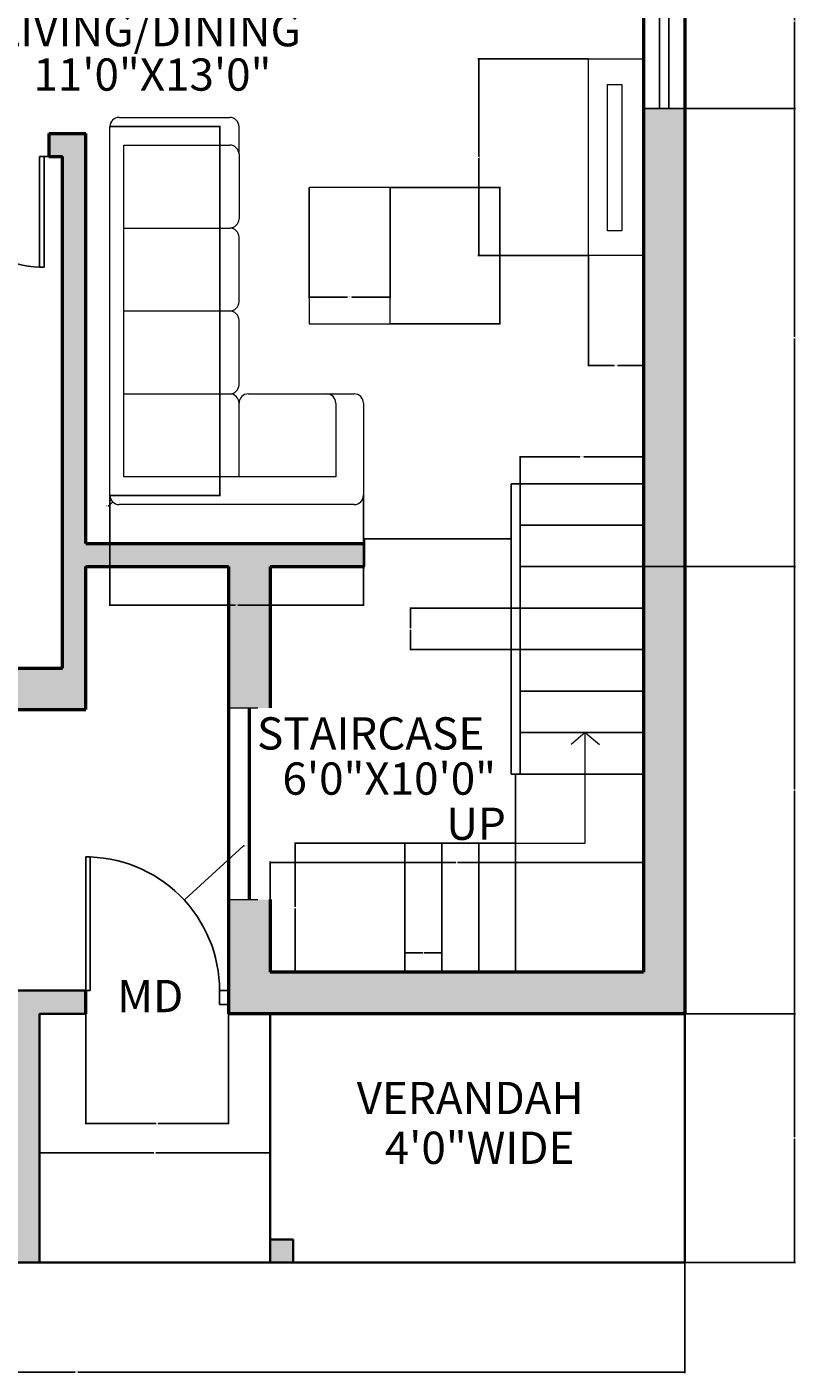
# Model space of a CAD drawing. Units: inches. Extents: x 2715 to 3027, y 1777 to 2287.
# Tile 2 of 4: x 2860 to 3027, y 1777 to 2069. Entities that reach past the tile are written whole.
import ezdxf

# ---------------------------------------------------------------- set-up
doc = ezdxf.new("R2010")
doc.units = ezdxf.units.IN
doc.linetypes.add('DASHED2', pattern=[9.525, 6.35, -3.175])
for name, color, linetype, lineweight in [('A-ANNO-DIMS', 2, 'Continuous', 18), ('A-ANNO-SYMB', 7, 'Continuous', 18), ('A-ANNO-TEXT', 2, 'Continuous', 18), ('A-AREA-IDEN', 2, 'Continuous', 18), ('A-DOOR', 111, 'Continuous', 25), ('A-EQPM', 57, 'Continuous', 18), ('A-FLOR-STRS', 7, 'Continuous', 25), ('A-FURN', 201, 'Continuous', 18), ('A-GLAZ', 40, 'Continuous', 25), ('A-WALL', 7, 'Continuous', 50), ('A-WALL-HIDN', 255, 'DASHED2', 18), ('A-WALL-PATT', 252, 'Continuous', 13), ('C-SITE', 7, 'Continuous', 35)]:
    doc.layers.add(name, color=color, linetype=linetype, lineweight=lineweight)
doc.styles.get("Standard").update_dxf_attribs({"font": 'arial.ttf'})
doc.dimstyles.get("Standard").update_dxf_attribs({"dimtxt": 0.18, "dimasz": 0.18, "dimexe": 0.18, "dimexo": 0.0625, "dimgap": 0.09, "dimtad": 0, "dimtih": 1, "dimtoh": 1, "dimdec": 4, "dimzin": 0, "dimdsep": 46, "dimtxsty": 'Standard', "dimcen": 0.09, "dimadec": 0, "dimazin": 0, "dimtfac": 1, "dimtdec": 4, "dimtofl": 0, "dimtmove": 0, "dimatfit": 3, "dimfxl": 1, "dimtolj": 1, "dimtzin": 0, "dimarcsym": 0})

# ---------------------------------------------------------------- blocks, each defined once
blk = doc.blocks.new('*D25')
at = {"layer": 'A-ANNO-DIMS', "color": 0, "lineweight": -2, "transparency": 16777216}
for p, q in [((2738.92, 1801.28), (2738.92, 1777.36)), ((3002.92, 1801.28), (3002.92, 1777.36)), ((2739.1, 1777.54), (2870.63, 1777.54)), ((3002.74, 1777.54), (2871.21, 1777.54))]:
    blk.add_line(p, q, dxfattribs=at)
at = {"layer": 'A-ANNO-DIMS', "color": 0, "transparency": 16777216}
for points in [[(2739.1, 1777.57), (2739.1, 1777.51), (2738.92, 1777.54)], [(3002.74, 1777.57), (3002.74, 1777.51), (3002.92, 1777.54)]]:
    blk.add_solid(points, dxfattribs=at)
at = {"layer": 'Defpoints', "color": 0, "transparency": 16777216}
for p in [(2738.92, 1801.34), (3002.92, 1801.34), (3002.92, 1777.54)]:
    blk.add_point(p, dxfattribs=at)
at = {"layer": 'A-ANNO-DIMS', "color": 0, "transparency": 16777216, "insert": (2870.92, 1777.54), "char_height": 0.18, "attachment_point": 5}
blk.add_mtext('\\A1;264', dxfattribs=at)
blk = doc.blocks.new('*D27')
at = {"layer": 'A-ANNO-DIMS', "color": 0, "lineweight": -2, "transparency": 16777216}
for p, q in [((3002.98, 1855.34), (3026.9, 1855.34)), ((3026.72, 1855.16), (3026.72, 1828.52)), ((3026.72, 1801.52), (3026.72, 1828.16)), ((3002.98, 1801.34), (3026.9, 1801.34))]:
    blk.add_line(p, q, dxfattribs=at)
at = {"layer": 'A-ANNO-DIMS', "color": 0, "transparency": 16777216}
for points in [[(3026.69, 1855.16), (3026.75, 1855.16), (3026.72, 1855.34)], [(3026.69, 1801.52), (3026.75, 1801.52), (3026.72, 1801.34)]]:
    blk.add_solid(points, dxfattribs=at)
at = {"layer": 'Defpoints', "color": 0, "transparency": 16777216}
for p in [(3002.92, 1855.34), (3026.72, 1855.34), (3002.92, 1801.34)]:
    blk.add_point(p, dxfattribs=at)
at = {"layer": 'A-ANNO-DIMS', "color": 0, "transparency": 16777216, "insert": (3026.72, 1828.34), "char_height": 0.18, "attachment_point": 5}
blk.add_mtext('\\A1;54', dxfattribs=at)
blk = doc.blocks.new('*D28')
at = {"layer": 'A-ANNO-DIMS', "color": 0, "lineweight": -2, "transparency": 16777216}
for p, q in [((2993.98, 1952.34), (3026.9, 1952.34)), ((3026.72, 1952.16), (3026.72, 1904.02)), ((3026.72, 1855.52), (3026.72, 1903.66)), ((3002.98, 1855.34), (3026.9, 1855.34))]:
    blk.add_line(p, q, dxfattribs=at)
at = {"layer": 'A-ANNO-DIMS', "color": 0, "transparency": 16777216}
for points in [[(3026.69, 1952.16), (3026.75, 1952.16), (3026.72, 1952.34)], [(3026.69, 1855.52), (3026.75, 1855.52), (3026.72, 1855.34)]]:
    blk.add_solid(points, dxfattribs=at)
at = {"layer": 'Defpoints', "color": 0, "transparency": 16777216}
for p in [(2993.92, 1952.34), (3026.72, 1952.34), (3002.92, 1855.34)]:
    blk.add_point(p, dxfattribs=at)
at = {"layer": 'A-ANNO-DIMS', "color": 0, "transparency": 16777216, "insert": (3026.72, 1903.84), "char_height": 0.18, "attachment_point": 5}
blk.add_mtext('\\A1;97', dxfattribs=at)
blk = doc.blocks.new('*D29')
at = {"layer": 'A-ANNO-DIMS', "color": 0, "lineweight": -2, "transparency": 16777216}
for p, q in [((3002.98, 2051.72), (3026.9, 2051.72)), ((3026.72, 2051.54), (3026.72, 2002.21)), ((3026.72, 1952.52), (3026.72, 2001.85)), ((2993.98, 1952.34), (3026.9, 1952.34))]:
    blk.add_line(p, q, dxfattribs=at)
at = {"layer": 'A-ANNO-DIMS', "color": 0, "transparency": 16777216}
for points in [[(3026.69, 2051.54), (3026.75, 2051.54), (3026.72, 2051.72)], [(3026.69, 1952.52), (3026.75, 1952.52), (3026.72, 1952.34)]]:
    blk.add_solid(points, dxfattribs=at)
at = {"layer": 'Defpoints', "color": 0, "transparency": 16777216}
for p in [(3002.92, 2051.72), (3026.72, 2051.72), (2993.92, 1952.34)]:
    blk.add_point(p, dxfattribs=at)
at = {"layer": 'A-ANNO-DIMS', "color": 0, "transparency": 16777216, "insert": (3026.72, 2002.03), "char_height": 0.18, "attachment_point": 5}
blk.add_mtext('\\A1;99.38', dxfattribs=at)
blk = doc.blocks.new('*D30')
at = {"layer": 'A-ANNO-DIMS', "color": 0, "lineweight": -2, "transparency": 16777216}
for p, q in [((3002.98, 2089.72), (3026.9, 2089.72)), ((3026.72, 2089.54), (3026.72, 2070.9)), ((3026.72, 2051.9), (3026.72, 2070.54)), ((3002.98, 2051.72), (3026.9, 2051.72))]:
    blk.add_line(p, q, dxfattribs=at)
at = {"layer": 'A-ANNO-DIMS', "color": 0, "transparency": 16777216}
for points in [[(3026.69, 2089.54), (3026.75, 2089.54), (3026.72, 2089.72)], [(3026.69, 2051.9), (3026.75, 2051.9), (3026.72, 2051.72)]]:
    blk.add_solid(points, dxfattribs=at)
at = {"layer": 'Defpoints', "color": 0, "transparency": 16777216}
for p in [(3002.92, 2089.72), (3026.72, 2089.72), (3002.92, 2051.72)]:
    blk.add_point(p, dxfattribs=at)
at = {"layer": 'A-ANNO-DIMS', "color": 0, "transparency": 16777216, "insert": (3026.72, 2070.72), "char_height": 0.18, "attachment_point": 5}
blk.add_mtext('\\A1;38', dxfattribs=at)
blk = doc.blocks.new('*D45')
at = {"layer": 'A-ANNO-DIMS', "color": 0, "lineweight": -2, "transparency": 16777216}
for p, q in [((2862.92, 1801.4), (2862.92, 1825.33)), ((2863.1, 1825.15), (2887.7, 1825.15)), ((2912.74, 1825.15), (2888.13, 1825.15)), ((2912.92, 1801.4), (2912.92, 1825.33))]:
    blk.add_line(p, q, dxfattribs=at)
at = {"layer": 'A-ANNO-DIMS', "color": 0, "transparency": 16777216}
for points in [[(2863.1, 1825.18), (2863.1, 1825.12), (2862.92, 1825.15)], [(2912.74, 1825.18), (2912.74, 1825.12), (2912.92, 1825.15)]]:
    blk.add_solid(points, dxfattribs=at)
at = {"layer": 'Defpoints', "color": 0, "transparency": 16777216}
for p in [(2912.92, 1825.15), (2862.92, 1801.34), (2912.92, 1801.34)]:
    blk.add_point(p, dxfattribs=at)
at = {"layer": 'A-ANNO-DIMS', "color": 0, "transparency": 16777216, "insert": (2887.92, 1825.15), "char_height": 0.18, "attachment_point": 5}
blk.add_mtext('\\A1;50', dxfattribs=at)
blk = doc.blocks.new('*D46')
at = {"layer": 'A-ANNO-DIMS', "color": 0, "lineweight": -2, "transparency": 16777216}
for p, q in [((2912.92, 1864.4), (2912.92, 1888.33)), ((2913.1, 1888.15), (2953.21, 1888.15)), ((2993.74, 1888.15), (2953.62, 1888.15)), ((2993.92, 1864.4), (2993.92, 1888.33))]:
    blk.add_line(p, q, dxfattribs=at)
at = {"layer": 'A-ANNO-DIMS', "color": 0, "transparency": 16777216}
for points in [[(2913.1, 1888.18), (2913.1, 1888.12), (2912.92, 1888.15)], [(2993.74, 1888.18), (2993.74, 1888.12), (2993.92, 1888.15)]]:
    blk.add_solid(points, dxfattribs=at)
at = {"layer": 'Defpoints', "color": 0, "transparency": 16777216}
for p in [(2993.92, 1888.15), (2912.92, 1864.34), (2993.92, 1864.34)]:
    blk.add_point(p, dxfattribs=at)
at = {"layer": 'A-ANNO-DIMS', "color": 0, "transparency": 16777216, "insert": (2953.42, 1888.15), "char_height": 0.18, "attachment_point": 5}
blk.add_mtext('\\A1;81', dxfattribs=at)
blk = doc.blocks.new('*D50')
at = {"layer": 'A-ANNO-DIMS', "color": 0, "lineweight": -2, "transparency": 16777216}
for p, q in [((2872.92, 1855.28), (2872.92, 1831.36)), ((2903.92, 1855.28), (2903.92, 1831.36)), ((2873.1, 1831.54), (2888.21, 1831.54)), ((2903.74, 1831.54), (2888.62, 1831.54))]:
    blk.add_line(p, q, dxfattribs=at)
at = {"layer": 'A-ANNO-DIMS', "color": 0, "transparency": 16777216}
for points in [[(2873.1, 1831.57), (2873.1, 1831.51), (2872.92, 1831.54)], [(2903.74, 1831.57), (2903.74, 1831.51), (2903.92, 1831.54)]]:
    blk.add_solid(points, dxfattribs=at)
at = {"layer": 'Defpoints', "color": 0, "transparency": 16777216}
for p in [(2872.92, 1855.34), (2903.92, 1855.34), (2872.92, 1831.54)]:
    blk.add_point(p, dxfattribs=at)
at = {"layer": 'A-ANNO-DIMS', "color": 0, "transparency": 16777216, "insert": (2888.42, 1831.54), "char_height": 0.18, "attachment_point": 5}
blk.add_mtext('\\A1;31', dxfattribs=at)
blk = doc.blocks.new('*D62')
at = {"layer": 'A-ANNO-DIMS', "color": 0, "lineweight": -2, "transparency": 16777216}
for p, q in [((2878.17, 1967.75), (2878.17, 1943.83)), ((2933.17, 1967.75), (2933.17, 1943.83)), ((2878.35, 1944.01), (2905.45, 1944.01)), ((2932.99, 1944.01), (2905.89, 1944.01))]:
    blk.add_line(p, q, dxfattribs=at)
at = {"layer": 'A-ANNO-DIMS', "color": 0, "transparency": 16777216}
for points in [[(2878.35, 1944.04), (2878.35, 1943.98), (2878.17, 1944.01)], [(2932.99, 1944.04), (2932.99, 1943.98), (2933.17, 1944.01)]]:
    blk.add_solid(points, dxfattribs=at)
at = {"layer": 'Defpoints', "color": 0, "transparency": 16777216}
for p in [(2878.17, 1967.81), (2933.17, 1967.81), (2878.17, 1944.01)]:
    blk.add_point(p, dxfattribs=at)
at = {"layer": 'A-ANNO-DIMS', "color": 0, "transparency": 16777216, "insert": (2905.67, 1944.01), "char_height": 0.18, "attachment_point": 5}
blk.add_mtext('\\A1;55', dxfattribs=at)
blk = doc.blocks.new('*D63')
at = {"layer": 'A-ANNO-DIMS', "color": 0, "lineweight": -2, "transparency": 16777216}
for p, q in [((2878.24, 2047.81), (2902.16, 2047.81)), ((2901.98, 2047.63), (2901.98, 2008)), ((2901.98, 1967.99), (2901.98, 2007.63)), ((2878.24, 1967.81), (2902.16, 1967.81))]:
    blk.add_line(p, q, dxfattribs=at)
at = {"layer": 'A-ANNO-DIMS', "color": 0, "transparency": 16777216}
for points in [[(2901.95, 2047.63), (2902.01, 2047.63), (2901.98, 2047.81)], [(2901.95, 1967.99), (2902.01, 1967.99), (2901.98, 1967.81)]]:
    blk.add_solid(points, dxfattribs=at)
at = {"layer": 'Defpoints', "color": 0, "transparency": 16777216}
for p in [(2878.17, 2047.81), (2878.17, 1967.81), (2901.98, 1967.81)]:
    blk.add_point(p, dxfattribs=at)
at = {"layer": 'A-ANNO-DIMS', "color": 0, "transparency": 16777216, "insert": (2901.98, 2007.81), "char_height": 0.18, "attachment_point": 5}
blk.add_mtext('\\A1;80', dxfattribs=at)
blk = doc.blocks.new('*D67')
at = {"layer": 'A-ANNO-DIMS', "color": 0, "lineweight": -2, "transparency": 16777216}
for p, q in [((2939.02, 2034.61), (2962.94, 2034.61)), ((2962.76, 2034.43), (2962.76, 2020.01)), ((2962.76, 2005.23), (2962.76, 2019.65)), ((2939.02, 2005.05), (2962.94, 2005.05))]:
    blk.add_line(p, q, dxfattribs=at)
at = {"layer": 'A-ANNO-DIMS', "color": 0, "transparency": 16777216}
for points in [[(2962.73, 2034.43), (2962.79, 2034.43), (2962.76, 2034.61)], [(2962.73, 2005.23), (2962.79, 2005.23), (2962.76, 2005.05)]]:
    blk.add_solid(points, dxfattribs=at)
at = {"layer": 'Defpoints', "color": 0, "transparency": 16777216}
for p in [(2938.95, 2034.61), (2938.95, 2005.05), (2962.76, 2005.05)]:
    blk.add_point(p, dxfattribs=at)
at = {"layer": 'A-ANNO-DIMS', "color": 0, "transparency": 16777216, "insert": (2962.76, 2019.83), "char_height": 0.18, "attachment_point": 5}
blk.add_mtext('\\A1;29.57', dxfattribs=at)
blk = doc.blocks.new('*D68')
at = {"layer": 'A-ANNO-DIMS', "color": 0, "lineweight": -2, "transparency": 16777216}
for p, q in [((2921.42, 2034.55), (2921.42, 2010.63)), ((2938.95, 2034.55), (2938.95, 2010.63)), ((2921.6, 2010.81), (2929.73, 2010.81)), ((2938.77, 2010.81), (2930.64, 2010.81))]:
    blk.add_line(p, q, dxfattribs=at)
at = {"layer": 'A-ANNO-DIMS', "color": 0, "transparency": 16777216}
for points in [[(2921.6, 2010.84), (2921.6, 2010.78), (2921.42, 2010.81)], [(2938.77, 2010.84), (2938.77, 2010.78), (2938.95, 2010.81)]]:
    blk.add_solid(points, dxfattribs=at)
at = {"layer": 'Defpoints', "color": 0, "transparency": 16777216}
for p in [(2921.42, 2034.61), (2938.95, 2034.61), (2921.42, 2010.81)]:
    blk.add_point(p, dxfattribs=at)
at = {"layer": 'A-ANNO-DIMS', "color": 0, "transparency": 16777216, "insert": (2930.19, 2010.81), "char_height": 0.18, "attachment_point": 5}
blk.add_mtext('\\A1;17.537', dxfattribs=at)
blk = doc.blocks.new('*D69')
at = {"layer": 'A-ANNO-DIMS', "color": 0, "lineweight": -2, "transparency": 16777216}
for p, q in [((2981.91, 2062.54), (2957.99, 2062.54)), ((2958.17, 2062.36), (2958.17, 2041.36)), ((2958.17, 2020.01), (2958.17, 2041)), ((2981.91, 2019.83), (2957.99, 2019.83))]:
    blk.add_line(p, q, dxfattribs=at)
at = {"layer": 'A-ANNO-DIMS', "color": 0, "transparency": 16777216}
for points in [[(2958.14, 2062.36), (2958.2, 2062.36), (2958.17, 2062.54)], [(2958.14, 2020.01), (2958.2, 2020.01), (2958.17, 2019.83)]]:
    blk.add_solid(points, dxfattribs=at)
at = {"layer": 'Defpoints', "color": 0, "transparency": 16777216}
for p in [(2958.17, 2062.54), (2981.97, 2062.54), (2981.97, 2019.83)]:
    blk.add_point(p, dxfattribs=at)
at = {"layer": 'A-ANNO-DIMS', "color": 0, "transparency": 16777216, "insert": (2958.17, 2041.18), "char_height": 0.18, "attachment_point": 5}
blk.add_mtext('\\A1;42.71', dxfattribs=at)
blk = doc.blocks.new('*D70')
at = {"layer": 'A-ANNO-DIMS', "color": 0, "lineweight": -2, "transparency": 16777216}
for p, q in [((2981.97, 2019.77), (2981.97, 1995.84)), ((2993.92, 2019.77), (2993.92, 1995.84)), ((2982.15, 1996.02), (2987.56, 1996.02)), ((2993.74, 1996.02), (2988.33, 1996.02))]:
    blk.add_line(p, q, dxfattribs=at)
at = {"layer": 'A-ANNO-DIMS', "color": 0, "transparency": 16777216}
for points in [[(2982.15, 1996.05), (2982.15, 1995.99), (2981.97, 1996.02)], [(2993.74, 1996.05), (2993.74, 1995.99), (2993.92, 1996.02)]]:
    blk.add_solid(points, dxfattribs=at)
at = {"layer": 'Defpoints', "color": 0, "transparency": 16777216}
for p in [(2981.97, 2019.83), (2993.92, 2019.83), (2981.97, 1996.02)]:
    blk.add_point(p, dxfattribs=at)
at = {"layer": 'A-ANNO-DIMS', "color": 0, "transparency": 16777216, "insert": (2987.95, 1996.02), "char_height": 0.18, "attachment_point": 5}
blk.add_mtext('\\A1;11.94', dxfattribs=at)
blk = doc.blocks.new('*D71')
at = {"layer": 'A-ANNO-DIMS', "color": 0, "lineweight": -2, "transparency": 16777216}
for p, q in [((2967.18, 1952.4), (2967.18, 1976.33)), ((2967.36, 1976.15), (2980.08, 1976.15)), ((2993.74, 1976.15), (2981.01, 1976.15)), ((2993.92, 1952.4), (2993.92, 1976.33))]:
    blk.add_line(p, q, dxfattribs=at)
at = {"layer": 'A-ANNO-DIMS', "color": 0, "transparency": 16777216}
for points in [[(2967.36, 1976.18), (2967.36, 1976.12), (2967.18, 1976.15)], [(2993.74, 1976.18), (2993.74, 1976.12), (2993.92, 1976.15)]]:
    blk.add_solid(points, dxfattribs=at)
at = {"layer": 'Defpoints', "color": 0, "transparency": 16777216}
for p in [(2993.92, 1976.15), (2967.18, 1952.34), (2993.92, 1952.34)]:
    blk.add_point(p, dxfattribs=at)
at = {"layer": 'A-ANNO-DIMS', "color": 0, "transparency": 16777216, "insert": (2980.55, 1976.15), "char_height": 0.18, "attachment_point": 5}
blk.add_mtext('\\A1;26.733', dxfattribs=at)
blk = doc.blocks.new('*D72')
at = {"layer": 'A-ANNO-DIMS', "color": 0, "lineweight": -2, "transparency": 16777216}
for p, q in [((2967.12, 1943.34), (2943.2, 1943.34)), ((2943.38, 1943.16), (2943.38, 1939.02)), ((2943.38, 1934.52), (2943.38, 1938.66)), ((2967.12, 1934.34), (2943.2, 1934.34))]:
    blk.add_line(p, q, dxfattribs=at)
at = {"layer": 'A-ANNO-DIMS', "color": 0, "transparency": 16777216}
for points in [[(2943.35, 1943.16), (2943.41, 1943.16), (2943.38, 1943.34)], [(2943.35, 1934.52), (2943.41, 1934.52), (2943.38, 1934.34)]]:
    blk.add_solid(points, dxfattribs=at)
at = {"layer": 'Defpoints', "color": 0, "transparency": 16777216}
for p in [(2943.38, 1943.34), (2967.18, 1943.34), (2967.18, 1934.34)]:
    blk.add_point(p, dxfattribs=at)
at = {"layer": 'A-ANNO-DIMS', "color": 0, "transparency": 16777216, "insert": (2943.38, 1938.84), "char_height": 0.18, "attachment_point": 5}
blk.add_mtext('\\A1;9', dxfattribs=at)
blk = doc.blocks.new('*D73')
at = {"layer": 'A-ANNO-DIMS', "color": 0, "lineweight": -2, "transparency": 16777216}
for p, q in [((2942.18, 1892.28), (2942.18, 1868.36)), ((2950.18, 1892.28), (2950.18, 1868.36)), ((2942.36, 1868.54), (2946.03, 1868.54)), ((2950, 1868.54), (2946.33, 1868.54))]:
    blk.add_line(p, q, dxfattribs=at)
at = {"layer": 'A-ANNO-DIMS', "color": 0, "transparency": 16777216}
for points in [[(2942.36, 1868.57), (2942.36, 1868.51), (2942.18, 1868.54)], [(2950, 1868.57), (2950, 1868.51), (2950.18, 1868.54)]]:
    blk.add_solid(points, dxfattribs=at)
at = {"layer": 'Defpoints', "color": 0, "transparency": 16777216}
for p in [(2942.18, 1892.34), (2950.18, 1892.34), (2942.18, 1868.54)]:
    blk.add_point(p, dxfattribs=at)
at = {"layer": 'A-ANNO-DIMS', "color": 0, "transparency": 16777216, "insert": (2946.18, 1868.54), "char_height": 0.18, "attachment_point": 5}
blk.add_mtext('\\A1;8', dxfattribs=at)
blk = doc.blocks.new('*D74')
at = {"layer": 'A-ANNO-DIMS', "color": 0, "lineweight": -2, "transparency": 16777216}
for p, q in [((2942.12, 1892.34), (2918.2, 1892.34)), ((2918.38, 1892.16), (2918.38, 1878.52)), ((2918.38, 1864.52), (2918.38, 1878.16)), ((2942.12, 1864.34), (2918.2, 1864.34))]:
    blk.add_line(p, q, dxfattribs=at)
at = {"layer": 'A-ANNO-DIMS', "color": 0, "transparency": 16777216}
for points in [[(2918.35, 1892.16), (2918.41, 1892.16), (2918.38, 1892.34)], [(2918.35, 1864.52), (2918.41, 1864.52), (2918.38, 1864.34)]]:
    blk.add_solid(points, dxfattribs=at)
at = {"layer": 'Defpoints', "color": 0, "transparency": 16777216}
for p in [(2918.38, 1892.34), (2942.18, 1892.34), (2942.18, 1864.34)]:
    blk.add_point(p, dxfattribs=at)
at = {"layer": 'A-ANNO-DIMS', "color": 0, "transparency": 16777216, "insert": (2918.38, 1878.34), "char_height": 0.18, "attachment_point": 5}
blk.add_mtext('\\A1;28', dxfattribs=at)
blk = doc.blocks.new('*D75')
at = {"layer": 'A-ANNO-DIMS', "color": 0, "lineweight": -2, "transparency": 16777216}
for p, q in [((2907.14, 1891.73), (2894.45, 1880.09)), ((2907.32, 1891.73), (2907.14, 1891.73)), ((2872.87, 1860.36), (2873.05, 1860.36)), ((2872.96, 1860.27), (2872.96, 1860.45))]:
    blk.add_line(p, q, dxfattribs=at)
at = {"layer": 'A-ANNO-DIMS', "color": 0, "transparency": 16777216}
blk.add_solid([(2894.43, 1880.11), (2894.47, 1880.07), (2894.32, 1879.97)], dxfattribs=at)
at = {"layer": 'Defpoints', "color": 0, "transparency": 16777216}
for p in [(2894.32, 1879.97), (2872.96, 1860.36)]:
    blk.add_point(p, dxfattribs=at)
at = {"layer": 'A-ANNO-DIMS', "color": 0, "transparency": 16777216, "insert": (2907.62, 1891.73), "char_height": 0.18, "attachment_point": 5}
blk.add_mtext('\\A1;R29', dxfattribs=at)
blk = doc.blocks.new('*D77')
at = {"layer": 'A-ANNO-DIMS', "color": 0, "lineweight": -2, "transparency": 16777216}
for p, q in [((2863.69, 2041.32), (2863.87, 2041.32)), ((2863.78, 2041.23), (2863.78, 2041.41)), ((2834.78, 2016.15), (2845.52, 2025.48)), ((2834.6, 2016.15), (2834.78, 2016.15))]:
    blk.add_line(p, q, dxfattribs=at)
at = {"layer": 'A-ANNO-DIMS', "color": 0, "transparency": 16777216}
blk.add_solid([(2845.5, 2025.5), (2845.54, 2025.45), (2845.66, 2025.59)], dxfattribs=at)
at = {"layer": 'Defpoints', "color": 0, "transparency": 16777216}
for p in [(2863.78, 2041.32), (2845.66, 2025.59)]:
    blk.add_point(p, dxfattribs=at)
at = {"layer": 'A-ANNO-DIMS', "color": 0, "transparency": 16777216, "insert": (2834.11, 2016.15), "char_height": 0.18, "attachment_point": 5}
blk.add_mtext('\\A1;3X R24', dxfattribs=at)
blk = doc.blocks.new('*D79')
at = {"layer": 'A-ANNO-DIMS', "color": 0, "lineweight": -2, "transparency": 16777216}
for p, q in [((2877.94, 1965.52), (2878.65, 1966.25)), ((2880.08, 1967.81), (2880.26, 1967.81)), ((2880.17, 1967.72), (2880.17, 1967.9)), ((2877.76, 1965.52), (2877.94, 1965.52))]:
    blk.add_line(p, q, dxfattribs=at)
at = {"layer": 'A-ANNO-DIMS', "color": 0, "transparency": 16777216}
blk.add_solid([(2878.63, 1966.27), (2878.68, 1966.23), (2878.78, 1966.38)], dxfattribs=at)
at = {"layer": 'Defpoints', "color": 0, "transparency": 16777216}
for p in [(2878.78, 1966.38), (2880.17, 1967.81)]:
    blk.add_point(p, dxfattribs=at)
at = {"layer": 'A-ANNO-DIMS', "color": 0, "transparency": 16777216, "insert": (2877.53, 1965.52), "char_height": 0.18, "attachment_point": 5}
blk.add_mtext('\\A1;R2', dxfattribs=at)

msp = doc.modelspace()

# ---------------------------------------------------------------- hatches: boundary and pattern name
at = {"layer": 'A-WALL-PATT'}
h = msp.add_hatch(color=256, dxfattribs=at)
h.dxf.hatch_style = 1
h.paths.add_polyline_path([(3002.9159, 2051.722), (2993.9159, 2051.722), (2993.9159, 2019.8298), (2993.9159, 1864.3404), (2912.9159, 1864.3404), (2912.9159, 1880.0932), (2903.9159, 1880.0932), (2903.9159, 1864.3404), (2903.9159, 1855.3404), (3002.9159, 1855.3404)])
h = msp.add_hatch(color=256, dxfattribs=at)
h.dxf.hatch_style = 1
h.paths.add_polyline_path([(2872.9159, 2046.3404), (2864.9159, 2046.3404), (2864.9159, 2041.3404), (2867.9159, 2041.3404), (2867.9159, 1930.3404), (2829.9565, 1930.3404), (2829.9565, 1921.3404), (2872.9159, 1921.3404), (2872.9159, 1952.3404), (2903.9159, 1952.3404), (2903.9159, 1921.6914), (2912.9159, 1921.6914), (2912.9159, 1952.3404), (2933.4159, 1952.3404), (2933.4159, 1957.3404), (2872.9159, 1957.3404)])
h = msp.add_hatch(color=256, dxfattribs=at)
h.dxf.hatch_style = 1
h.paths.add_polyline_path([(2862.9159, 1855.3404), (2872.9159, 1855.3404), (2872.9159, 1860.3404), (2857.9159, 1860.3404), (2857.9159, 1806.3404), (2852.094, 1806.3404), (2852.094, 1801.3404), (2857.9159, 1801.3404), (2862.9159, 1801.3404)])
h = msp.add_hatch(color=256, dxfattribs=at)
h.dxf.hatch_style = 1
h.paths.add_polyline_path([(2917.9159, 1806.3404), (2912.9159, 1806.3404), (2912.9159, 1801.3404), (2917.9159, 1801.3404)])

# ---------------------------------------------------------------- linework, layer by layer
at = {"layer": 'A-ANNO-SYMB'}
for p, q in [((2981.2868, 1916.3404), (2978.2226, 1913.7692)), ((2981.2868, 1892.3404), (2981.2868, 1916.3404)), ((2981.2868, 1916.3404), (2984.3509, 1913.7692)), ((2966.1833, 1892.3404), (2981.2868, 1892.3404))]:
    msp.add_line(p, q, dxfattribs=at)
at = {"layer": 'A-DOOR'}
for p, q in [((2862.9159, 2017.3404), (2862.9159, 2041.3404)), ((2862.9159, 2041.3404), (2863.9159, 2041.3404)), ((2864.9159, 2041.3404), (2863.9159, 2041.3404)), ((2863.9159, 2041.3404), (2863.9159, 2017.3404)), ((2863.9159, 2017.3404), (2862.9159, 2017.3404)), ((2872.9159, 1860.3404), (2872.9159, 1889.3404)), ((2872.9159, 1889.3404), (2873.9159, 1889.3404)), ((2873.9159, 1889.3404), (2873.9159, 1860.3404)), ((2873.9159, 1860.3404), (2872.9159, 1860.3404)), ((2901.9159, 1860.3404), (2903.9159, 1860.3404)), ((2901.9159, 1857.3404), (2901.9159, 1860.3404)), ((2903.9159, 1860.3404), (2903.9159, 1857.3404)), ((2903.9159, 1857.3404), (2901.9159, 1857.3404))]:
    msp.add_line(p, q, dxfattribs=at)
for centre, radius, start, end in [((2863.7837, 2041.3247), 24, 173.983171, 267.927858), ((2872.9556, 1860.3563), 29, 357.003634, 88.102268)]:
    msp.add_arc(centre, radius, start, end, dxfattribs=at)
at = {"layer": 'A-EQPM'}
for points in [[(2993.9159, 2019.8298), (2981.9748, 2019.8298), (2981.9748, 2062.5394), (2993.9159, 2062.5394)], [(2986.1209, 2056.9761), (2989.2138, 2056.9761), (2989.2138, 2025.2154), (2986.1209, 2025.2154)]]:
    msp.add_lwpolyline(points, close=True, dxfattribs=at)
at = {"layer": 'A-FLOR-STRS'}
for p, q in [((2965.1833, 1970.3404), (2993.9159, 1970.3404)), ((2965.1833, 1970.3404), (2965.1833, 1907.3404)), ((2967.1833, 1970.3404), (2967.1833, 1907.3404)), ((2967.1833, 1961.3404), (2993.9159, 1961.3404)), ((2933.4159, 1957.3404), (2933.4159, 1958.3404)), ((2933.4159, 1958.3404), (2965.1833, 1958.3404)), ((2967.1833, 1952.3404), (2993.9159, 1952.3404)), ((2967.1833, 1943.3404), (2993.9159, 1943.3404)), ((2967.1833, 1934.3404), (2993.9159, 1934.3404)), ((2967.1833, 1925.3404), (2993.9159, 1925.3404)), ((2967.1833, 1916.3404), (2993.9159, 1916.3404)), ((2965.1833, 1907.3404), (2993.9159, 1907.3404)), ((2966.1833, 1892.3404), (2966.1833, 1907.3404)), ((2942.1833, 1864.3404), (2942.1833, 1892.3404)), ((2942.1833, 1892.3404), (2966.1833, 1892.3404)), ((2950.1833, 1864.3404), (2950.1833, 1892.3404)), ((2958.1833, 1864.3404), (2958.1833, 1892.3404)), ((2966.1833, 1864.3404), (2966.1833, 1892.3404))]:
    msp.add_line(p, q, dxfattribs=at)
at = {"layer": 'A-FURN'}
for p, q in [((2878.1746, 1967.8133), (2878.1746, 2047.8133)), ((2880.1746, 2049.8133), (2904.1746, 2049.8133)), ((2906.1746, 2041.8133), (2906.1746, 2047.8133)), ((2881.1746, 2043.8133), (2904.1746, 2043.8133)), ((2881.1746, 1971.8133), (2881.1746, 2043.8133)), ((2906.1746, 2041.8133), (2906.1746, 2027.8133)), ((2881.1746, 2025.8133), (2904.1746, 2025.8133)), ((2904.1746, 2025.8133), (2904.1746, 2025.8133)), ((2906.1746, 2009.8133), (2906.1746, 2023.8133)), ((2881.1746, 2007.8133), (2904.1746, 2007.8133)), ((2904.1746, 2007.8133), (2904.1746, 2007.8133)), ((2906.1746, 1991.8133), (2906.1746, 2005.8133)), ((2881.1746, 1989.8133), (2904.1746, 1989.8133)), ((2904.1746, 1989.8133), (2904.1746, 1989.8133)), ((2908.1746, 1989.8133), (2925.1746, 1989.8133)), ((2925.1746, 1989.8133), (2931.1746, 1989.8133)), ((2906.1746, 1971.8133), (2906.1746, 1987.8133)), ((2906.1746, 1987.8133), (2906.1746, 1987.8133)), ((2927.1746, 1987.8133), (2927.1746, 1971.8133)), ((2933.1746, 1987.8133), (2933.1746, 1967.8133)), ((2906.1746, 1971.8133), (2881.1746, 1971.8133)), ((2927.1746, 1971.8133), (2906.1746, 1971.8133)), ((2906.1746, 1965.8133), (2880.1746, 1965.8133)), ((2931.1746, 1965.8133), (2906.1746, 1965.8133))]:
    msp.add_line(p, q, dxfattribs=at)
msp.add_lwpolyline([(2921.4175, 2005.0458), (2938.9545, 2005.0458), (2938.9545, 2034.6139), (2921.4175, 2034.6139)], close=True, dxfattribs=at)
for centre, start, end in [((2880.1746, 2047.8133), 90, 180), ((2904.1746, 2047.8133), 0, 90), ((2904.1746, 2041.8133), 0, 90), ((2904.1746, 2027.8133), 270, 0), ((2904.1746, 2023.8133), 0, 90), ((2904.1746, 2009.8133), 270, 0), ((2904.1746, 2005.8133), 0, 90), ((2904.1746, 1991.8133), 270, 0), ((2904.1746, 1987.8133), 0, 90), ((2908.1746, 1987.8133), 90, 180), ((2925.1746, 1987.8133), 0, 90), ((2931.1746, 1987.8133), 0, 90), ((2880.1746, 1967.8133), 180, 270), ((2931.1746, 1967.8133), 270, 0)]:
    msp.add_arc(centre, 2, start, end, dxfattribs=at)
at = {"layer": 'A-GLAZ'}
for p, q in [((2997.4159, 2089.722), (2997.4159, 2051.722)), ((2999.4159, 2089.722), (2999.4159, 2051.722)), ((2993.9159, 2051.722), (3002.9159, 2051.722))]:
    msp.add_line(p, q, dxfattribs=at)
at = {"layer": 'A-WALL'}
for p, q in [((2993.9159, 2141.3404), (2993.9159, 1864.3404)), ((2864.9159, 2046.3404), (2864.9159, 2041.3404)), ((2864.9159, 2046.3404), (2872.9159, 2046.3404)), ((2872.9159, 1957.3404), (2872.9159, 2046.3404)), ((2864.9159, 2041.3404), (2867.9159, 2041.3404)), ((2867.9159, 1930.3404), (2867.9159, 2041.3404)), ((2872.9159, 1957.3404), (2933.4159, 1957.3404)), ((2872.9159, 1952.3404), (2903.9159, 1952.3404)), ((2872.9159, 1921.3404), (2872.9159, 1952.3404)), ((2903.9159, 1952.3404), (2903.9159, 1864.3404)), ((2912.9159, 1952.3404), (2912.9159, 1921.6914)), ((2912.9159, 1952.3404), (2933.4159, 1952.3404)), ((2747.9159, 1930.3404), (2867.9159, 1930.3404)), ((2738.9159, 1921.3404), (2872.9159, 1921.3404)), ((2908.4159, 1880.0932), (2908.4159, 1921.6914)), ((2912.9159, 1880.0932), (2912.9159, 1864.3404)), ((2903.9159, 1864.3404), (2903.9159, 1855.3404)), ((2993.9159, 1864.3404), (2912.9159, 1864.3404)), ((2872.9159, 1855.3404), (2872.9159, 1860.3404))]:
    msp.add_line(p, q, dxfattribs=at)
msp.add_lwpolyline([(2738.9159, 1921.3404), (2738.9159, 2263.3404), (3002.9159, 2263.3404), (3002.9159, 1855.3404), (2903.9159, 1855.3404)], dxfattribs=at)
at = {"layer": 'A-WALL-HIDN'}
for p, q in [((2933.4159, 1957.3404), (2933.4159, 1952.3404)), ((2903.9159, 1921.6914), (2912.9159, 1921.6914)), ((2903.9159, 1880.0932), (2912.9159, 1880.0932))]:
    msp.add_line(p, q, dxfattribs=at)
at = {"layer": 'C-SITE'}
for p, q in [((2872.9159, 1860.3404), (2857.9159, 1860.3404)), ((2862.9159, 1801.3404), (2862.9159, 1855.3404)), ((2862.9159, 1855.3404), (2872.9159, 1855.3404)), ((2912.9159, 1855.3404), (2912.9159, 1801.3404)), ((3002.9159, 1801.3404), (3002.9159, 1855.3404)), ((2912.9159, 1801.3404), (2912.9159, 1806.3404)), ((2912.9159, 1806.3404), (2917.9159, 1806.3404)), ((2917.9159, 1806.3404), (2917.9159, 1801.3404)), ((2857.9159, 1801.3404), (2862.9159, 1801.3404)), ((2862.9159, 1801.3404), (3002.9159, 1801.3404))]:
    msp.add_line(p, q, dxfattribs=at)

# ---------------------------------------------------------------- texts
at = {"layer": 'A-ANNO-SYMB'}
msp.add_attdef('UP', (2951.1375, 1893.0613), '', height=7, dxfattribs=at)
at = {"layer": 'A-ANNO-TEXT'}
msp.add_attdef('MD', (2879.7664, 1855.6631), '', height=7, dxfattribs=at)
at = {"layer": 'A-AREA-IDEN'}
for tag, p in [('LIVING/DINING', (2853.5433, 2065.2489)), ('11\'0"X13\'0"', (2861.5754, 2055.6187)), ('STAIRCASE', (2910.09, 1912.6537)), ('6\'0"X10\'0"', (2915.6008, 1902.8522)), ('VERANDAH', (2931.7067, 1833.5468)), ('4\'0"WIDE', (2937.793, 1822.736))]:
    msp.add_attdef(tag, p, '', height=7, dxfattribs=at)

# ---------------------------------------------------------------- dimensions: what is measured, and where the dimension line sits
at = {"layer": 'A-ANNO-DIMS'}
for base, p1, p2, angle, override, picture, middle in [((3026.7209, 2089.722), (3002.9159, 2051.722), (3002.9159, 2089.722), 90, {"dimdec": 0, "dimlfac": 1, "dimrnd": 0, "dimzin": 0, "dimdsep": 46, "dimlunit": 2}, '*D30', (3026.7209, 2070.722)), ((2958.1698, 2062.5394), (2981.9748, 2019.8298), (2981.9748, 2062.5394), 90, {"dimdec": 2, "dimlfac": 1, "dimrnd": 0, "dimzin": 0, "dimdsep": 46, "dimlunit": 2}, '*D69', (2958.1698, 2041.1846)), ((3026.7209, 2051.722), (2993.9159, 1952.3404), (3002.9159, 2051.722), 90, {"dimdec": 2, "dimlfac": 1, "dimrnd": 0, "dimzin": 0, "dimdsep": 46, "dimlunit": 2}, '*D29', (3026.7209, 2002.0312)), ((2901.9796, 1967.8133), (2878.1746, 2047.8133), (2878.1746, 1967.8133), 270, {"dimdec": 0, "dimlfac": 1, "dimrnd": 0, "dimzin": 0, "dimdsep": 46, "dimlunit": 2}, '*D63', (2901.9796, 2007.8133)), ((2921.4175, 2010.8089), (2938.9545, 2034.6139), (2921.4175, 2034.6139), 180, {"dimdec": 3, "dimlfac": 1, "dimrnd": 0, "dimzin": 0, "dimdsep": 46, "dimlunit": 2}, '*D68', (2930.186, 2010.8089)), ((2962.7595, 2005.0458), (2938.9545, 2034.6139), (2938.9545, 2005.0458), 270, {"dimdec": 2, "dimlfac": 1, "dimrnd": 0, "dimzin": 0, "dimdsep": 46, "dimlunit": 2}, '*D67', (2962.7595, 2019.8298)), ((2981.9748, 1996.0248), (2993.9159, 2019.8298), (2981.9748, 2019.8298), 180, {"dimdec": 2, "dimlfac": 1, "dimrnd": 0, "dimzin": 0, "dimdsep": 46, "dimlunit": 2}, '*D70', (2987.9454, 1996.0248)), ((2993.9159, 1976.1454), (2967.1833, 1952.3404), (2993.9159, 1952.3404), 0, {"dimdec": 3, "dimlfac": 1, "dimrnd": 0, "dimzin": 0, "dimdsep": 46, "dimlunit": 2}, '*D71', (2980.5496, 1976.1454)), ((2878.1746, 1944.0083), (2933.1746, 1967.8133), (2878.1746, 1967.8133), 180, {"dimdec": 0, "dimlfac": 1, "dimrnd": 0, "dimzin": 0, "dimdsep": 46, "dimlunit": 2}, '*D62', (2905.6746, 1944.0083)), ((3026.7209, 1952.3404), (3002.9159, 1855.3404), (2993.9159, 1952.3404), 90, {"dimdec": 0, "dimlfac": 1, "dimrnd": 0, "dimzin": 0, "dimdsep": 46, "dimlunit": 2}, '*D28', (3026.7209, 1903.8404)), ((2943.3783, 1943.3404), (2967.1833, 1934.3404), (2967.1833, 1943.3404), 90, {"dimdec": 0, "dimlfac": 1, "dimrnd": 0, "dimzin": 0, "dimdsep": 46, "dimlunit": 2}, '*D72', (2943.3783, 1938.8404)), ((2918.3783, 1892.3404), (2942.1833, 1864.3404), (2942.1833, 1892.3404), 90, {"dimdec": 0, "dimlfac": 1, "dimrnd": 0, "dimzin": 0, "dimdsep": 46, "dimlunit": 2}, '*D74', (2918.3783, 1878.3404)), ((2942.1833, 1868.5354), (2950.1833, 1892.3404), (2942.1833, 1892.3404), 180, {"dimdec": 0, "dimlfac": 1, "dimrnd": 0, "dimzin": 0, "dimdsep": 46, "dimlunit": 2}, '*D73', (2946.1833, 1868.5354)), ((2872.9159, 1831.5354), (2903.9159, 1855.3404), (2872.9159, 1855.3404), 180, {"dimdec": 0, "dimlfac": 1, "dimrnd": 0, "dimzin": 0, "dimdsep": 46, "dimlunit": 2}, '*D50', (2888.4159, 1831.5354)), ((3026.7209, 1855.3404), (3002.9159, 1801.3404), (3002.9159, 1855.3404), 90, {"dimdec": 0, "dimlfac": 1, "dimrnd": 0, "dimzin": 0, "dimdsep": 46, "dimlunit": 2}, '*D27', (3026.7209, 1828.3404))]:
    dim = msp.add_linear_dim(base=base, p1=p1, p2=p2, angle=angle, dimstyle='Standard', override=override, dxfattribs=at)
    dim.commit()
    dim.dimension.update_dxf_attribs({"geometry": picture, "text_midpoint": middle})
dim = msp.add_radius_dim(center=(2863.7837, 2041.3247), mpoint=(2845.6584, 2025.5934), text='3X <>', dimstyle='Standard', override={"dimdec": 0, "dimlfac": 1, "dimrnd": 0, "dimzin": 0, "dimdsep": 46, "dimlunit": 2}, dxfattribs=at)
dim.commit()
dim.dimension.update_dxf_attribs({"geometry": '*D77', "text_midpoint": (2834.1053, 2016.1546), "dimtype": 164})
for center, mpoint, picture, middle in [((2880.1746, 1967.8133), (2878.7802, 1966.3796), '*D79', (2877.5293, 1965.5194)), ((2872.9556, 1860.3563), (2894.3188, 1879.9678), '*D75', (2907.622, 1891.7348))]:
    dim = msp.add_radius_dim(center=center, mpoint=mpoint, dimstyle='Standard', override={"dimdec": 0, "dimlfac": 1, "dimrnd": 0, "dimzin": 0, "dimdsep": 46, "dimlunit": 2}, dxfattribs=at)
    dim.commit()
    dim.dimension.update_dxf_attribs({"geometry": picture, "text_midpoint": middle, "dimtype": 164})
for base, p1, p2, picture, middle in [((2993.9159, 1888.1454), (2912.9159, 1864.3404), (2993.9159, 1864.3404), '*D46', (2953.4159, 1888.1454)), ((2912.9159, 1825.1454), (2862.9159, 1801.3404), (2912.9159, 1801.3404), '*D45', (2887.9159, 1825.1454)), ((3002.9159, 1777.5354), (2738.9159, 1801.3404), (3002.9159, 1801.3404), '*D25', (2870.9159, 1777.5354))]:
    dim = msp.add_linear_dim(base=base, p1=p1, p2=p2, dimstyle='Standard', override={"dimdec": 0, "dimlfac": 1, "dimrnd": 0, "dimzin": 0, "dimdsep": 46, "dimlunit": 2}, dxfattribs=at)
    dim.commit()
    dim.dimension.update_dxf_attribs({"geometry": picture, "text_midpoint": middle})

doc.saveas('drawing.dxf')
